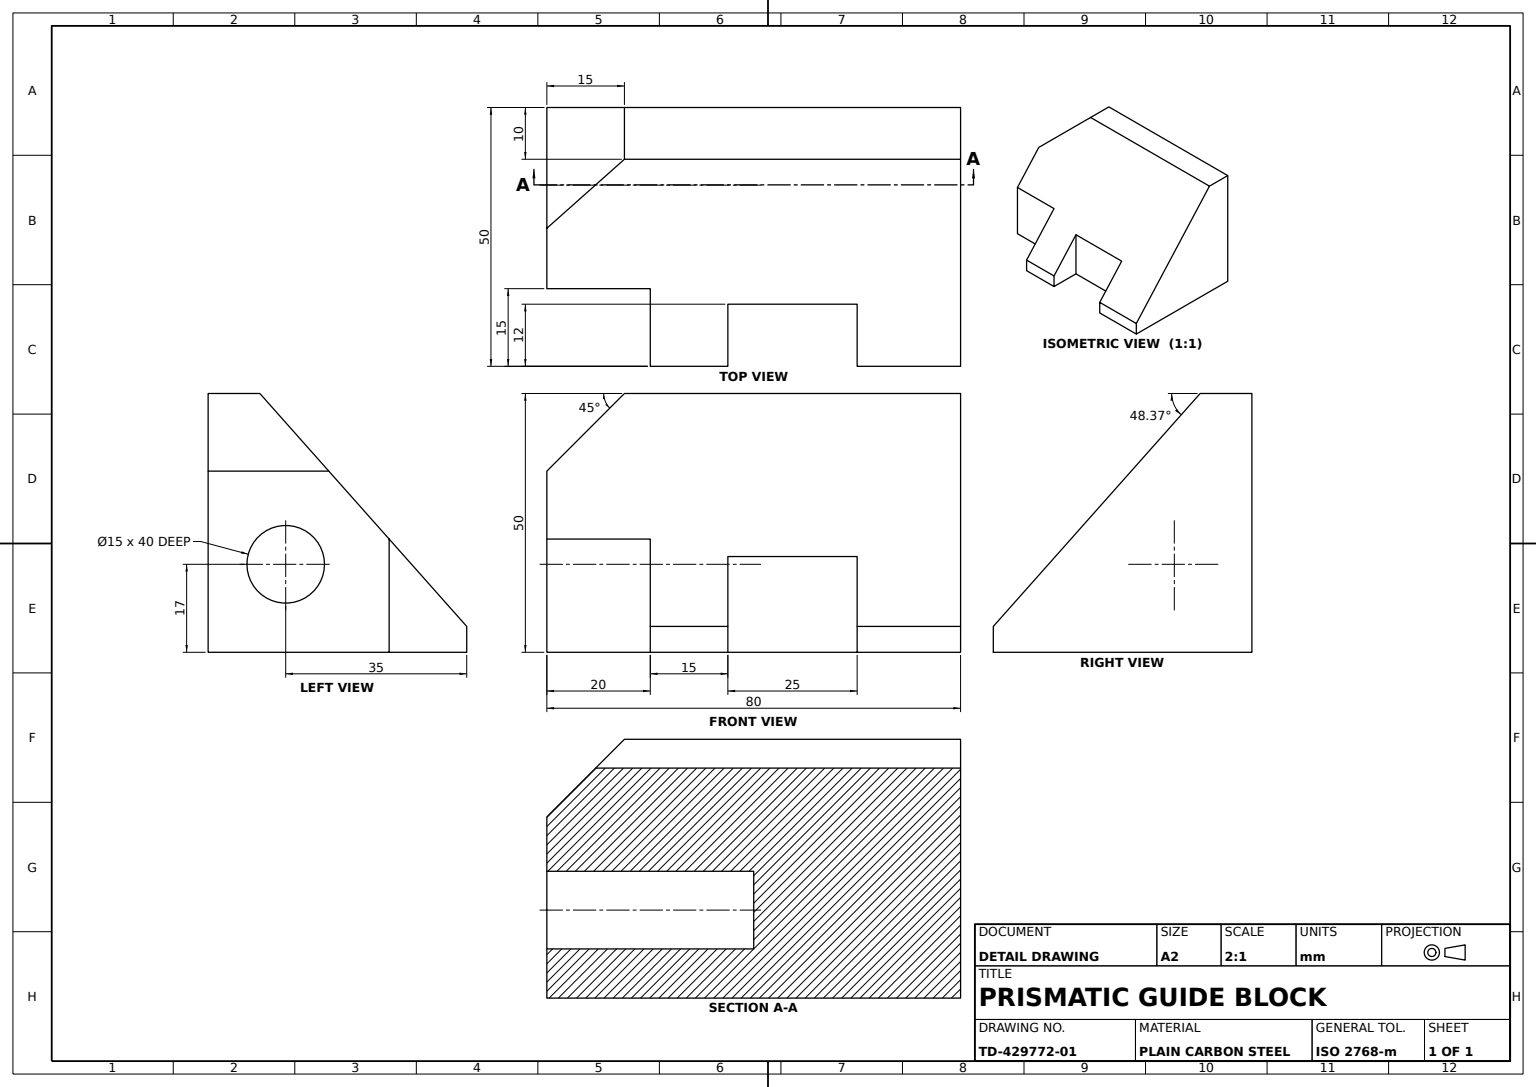
SolidWorks part; units mm, degrees
material "Plain Carbon Steel"
ref_plane "Front Plane" through (0, 0, 0) normal (0, 0, 1) x (1, 0, 0)
ref_plane "Top Plane" through (0, 0, 0) normal (0, 1, 0) x (1, 0, 0)
ref_plane "Right Plane" through (0, 0, 0) normal (1, 0, 0) x (0, 0, -1)
sketch "Bracket Profile Sketch" plane through (0, 0, 0) normal (0, 0, 1) x (1, 0, 0)
  line L0 (0, 0) -> (50, 0)
  line L1 (50, 0) -> (50, 5)
  line L2 (50, 5) -> (10, 50)
  line L3 (10, 50) -> (0, 50)
  line L4 (0, 50) -> (0, 0)
  line L5 (10, 50) -> (33.8367, 50) construction
  dimension "D1" = 50
  dimension "D2" = 50
  dimension "D3" = 48.366
  dimension "D4" = 10
extrude "Bracket Body" add sketch "Bracket Profile Sketch" along normal blind 80
sketch "Base Notch Sketch" plane through (0, 0, 0) normal (0, -1, 0) x (1, 0, 0)
  line L0 (50, 80) -> (50, 0) construction
  line L1 (50, 80) -> (35, 80)
  line L2 (50, 80) -> (50, 60)
  line L3 (50, 60) -> (35, 60)
  line L4 (35, 80) -> (35, 60)
  line L5 (50, 45) -> (38, 45)
  line L6 (50, 45) -> (50, 20)
  line L7 (50, 20) -> (38, 20)
  line L8 (38, 45) -> (38, 20)
  line L9 (0, 0) -> (50, 0) construction
  dimension "D1" = 15
  dimension "D2" = 20
  dimension "D3" = 20
  dimension "D4" = 25
  dimension "D5" = 12
extrude "Base Notch Cut" cut sketch "Base Notch Sketch" against normal blind 80
sketch "Side Hole Sketch" plane through (0, 0, 80) normal (0, 0, 1) x (1, 0, 0)
  line L0 (0, 0) -> (35, 0) construction
  line L1 (0, 50) -> (0, 0) construction
  circle A0 centre (15, 17) radius 7.5
  dimension "D3" = 15
  dimension "D1" = 17
  dimension "D2" = 15
extrude "Side Hole" cut sketch "Side Hole Sketch" against normal blind 40
sketch "Bevel Split Line Sketch" plane through (0, 0, 80) normal (0, 0, 1) x (1, 0, 0)
  line L0 (0, 35) -> (23.3333, 35)
  line L1 (0, 50) -> (0, 0) construction
  line L2 (35, 21.875) -> (10, 50) construction
  line L3 (10, 50) -> (0, 50) construction
  dimension "D1" = 15
split line "Bevel Split Line"
sketch "Half-Length Bevel Sketch" plane through (0, 0, 0) normal (-1, 0, 0) x (0, 0, 1)
  line L0 (80, 35) -> (65, 50)
  line L1 (80, 50) -> (0, 50) construction
  line L2 (65, 50) -> (80, 50)
  line L3 (80, 50) -> (80, 35) construction
  line L4 (80, 50) -> (80, 35)
extrude "Half-Length Bevel Cut" cut sketch "Half-Length Bevel Sketch" against normal blind 40
